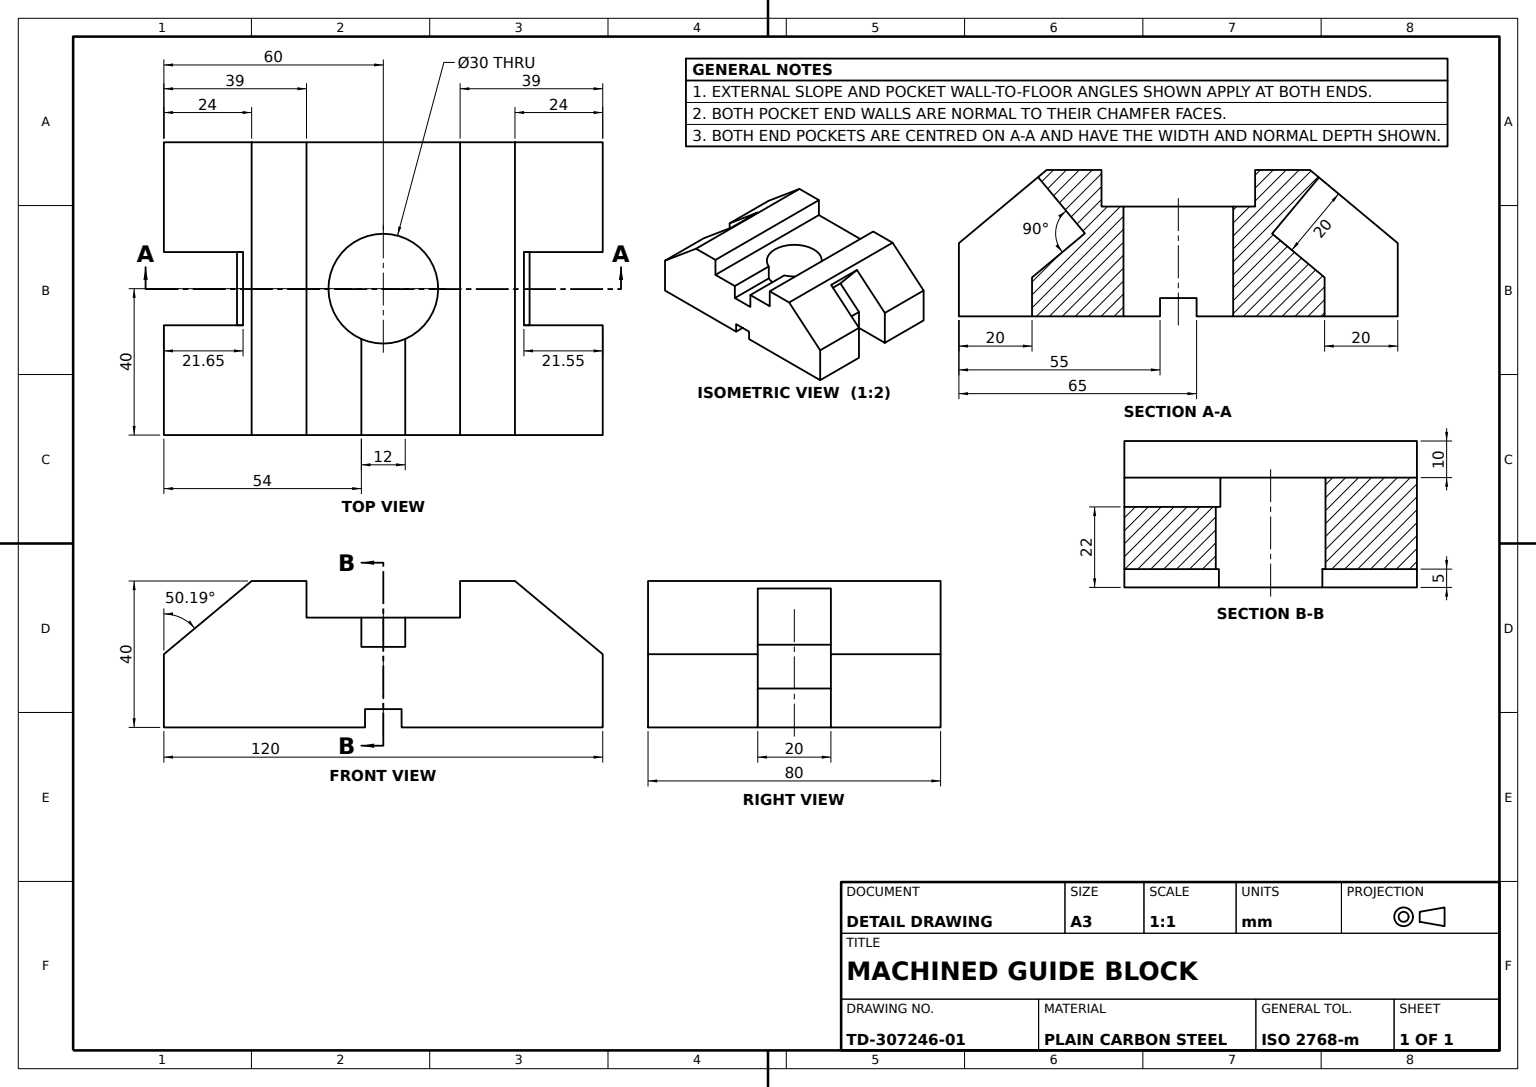
SolidWorks part; units mm, degrees
material "Plain Carbon Steel"
ref_plane "Front Plane" through (0, 0, 0) normal (0, 0, 1) x (1, 0, 0)
ref_plane "Top Plane" through (0, 0, 0) normal (0, 1, 0) x (1, 0, 0)
ref_plane "Right Plane" through (0, 0, 0) normal (1, 0, 0) x (0, 0, -1)
sketch "Block Profile Sketch" plane through (0, 0, 0) normal (0, 0, 1) x (1, 0, 0)
  line L0 (0, 0) -> (0, 20)
  line L1 (0, 0) -> (55, 0)
  line L2 (55, 0) -> (55, 5)
  line L3 (55, 5) -> (65, 5)
  line L4 (65, 5) -> (65, 0)
  line L5 (65, 0) -> (120, 0)
  line L6 (120, 0) -> (120, 20)
  line L7 (54, 30) -> (66, 30)
  line L10 (54, 30) -> (39, 30)
  line L11 (39, 30) -> (39, 40)
  line L12 (39, 40) -> (24, 40)
  line L13 (24, 40) -> (0, 20)
  line L16 (66, 30) -> (81, 30)
  line L17 (81, 30) -> (81, 40)
  line L18 (81, 40) -> (96, 40)
  line L19 (96, 40) -> (120, 20)
  dimension "D1" = 24
  dimension "D2" = 39
  dimension "D3" = 55
  dimension "D4" = 65
  dimension "D5" = 5
  dimension "D6" = 20
  dimension "D7" = 30
extrude "Block Body Extrude 80" add sketch "Block Profile Sketch" along normal blind 80
sketch "Through Cut Sketch" plane through (0, 30, 0) normal (0, 1, 0) x (1, 0, 0)
  line L0 (39, 0) -> (81, 0)
  line L1 (39, -80) -> (39, 0) construction
  line L3 (81, -80) -> (39, -80) construction
  circle A0 centre (60, -40) radius 15
  dimension "D1" = 30
  dimension "D4" = 30
  dimension "D2" = 21
  dimension "D3" = 40
extrude "Through Cut 80" cut sketch "Through Cut Sketch" against normal blind 80 contours A0
sketch "Profile Cut Sketch" plane through (0, 0, 80) normal (0, 0, 1) x (1, 0, 0)
  line L0 (60, 30) -> (66, 30)
  line L1 (81, 30) -> (39, 30) construction
  line L2 (60, 30) -> (54, 30)
  line L3 (54, 30) -> (54, 22)
  line L4 (54, 22) -> (66, 22)
  line L5 (66, 22) -> (66, 30)
  line L6 (120, 0) -> (120, 20) construction
  line L7 (65, 0) -> (120, 0) construction
  dimension "D1" = 54
  dimension "D2" = 22
extrude "Profile Cut 30" cut sketch "Profile Cut Sketch" against normal blind 30
sketch "Pocket A Sketch 30x30" plane through (120, 0, 0) normal (1, 0, 0) x (0, 0, -1)
  line L0 (-80, 20) -> (0, 20) construction
  line L1 (-50, 20) -> (-30, 20)
  line L2 (-50, 20) -> (-50, 0)
  line L3 (-50, 0) -> (-30, 0)
  line L4 (-30, 20) -> (-30, 0)
  line L5 (-80, 0) -> (0, 0) construction
  line L7 (-80, 0) -> (-80, 20) construction
  line L8 (0, 0) -> (0, 20) construction
  dimension "D1" = 30
  dimension "D2" = 30
extrude "Square Pocket A 30x30x20" cut sketch "Pocket A Sketch 30x30" against normal blind 20
sketch "Pocket A Extension Sketch" plane through (59.0164, 70.8197, 0) normal (0.6402, 0.7682, 0) x (0.7682, -0.6402, 0)
  line L0 (48.1419, -80) -> (48.1419, 0) construction
  line L1 (79.3829, -30) -> (79.3829, -50)
  line L2 (79.3829, -50) -> (51.3326, -50)
  line L3 (51.3326, -50) -> (51.3326, -30)
  line L4 (51.3326, -30) -> (79.3829, -30)
  dimension "D1" = 3.1908
extrude "Pocket A Extension Cut 20" cut sketch "Pocket A Extension Sketch" against normal blind 20
sketch "Pocket B Sketch 30x30" plane through (0, 0, 0) normal (-1, 0, 0) x (0, 0, 1)
  line L0 (80, 20) -> (0, 20) construction
  line L1 (30, 20) -> (50, 20)
  line L2 (30, 20) -> (30, 0)
  line L3 (30, 0) -> (50, 0)
  line L4 (50, 20) -> (50, 0)
  line L5 (80, 0) -> (0, 0) construction
  line L6 (80, 20) -> (80, 0) construction
  line L7 (0, 20) -> (0, 0) construction
  dimension "D1" = 30
  dimension "D2" = 30
extrude "Square Pocket B 30x30x20" cut sketch "Pocket B Sketch 30x30" against normal blind 20
sketch "Pocket B Extension Sketch" plane through (-9.8361, 11.8033, 0) normal (-0.6402, 0.7682, 0) x (0.7682, 0.6402, 0)
  line L0 (12.8037, -30) -> (40.9856, -30)
  line L1 (40.9856, -30) -> (40.9856, -50)
  line L2 (40.9856, -50) -> (12.8037, -50)
  line L3 (12.8037, -50) -> (12.8037, -30)
  line L5 (12.8037, -30) -> (12.8037, 0) construction
  dimension "D1" = 28.1819
extrude "Pocket B Extension Cut 20" cut sketch "Pocket B Extension Sketch" against normal blind 20
